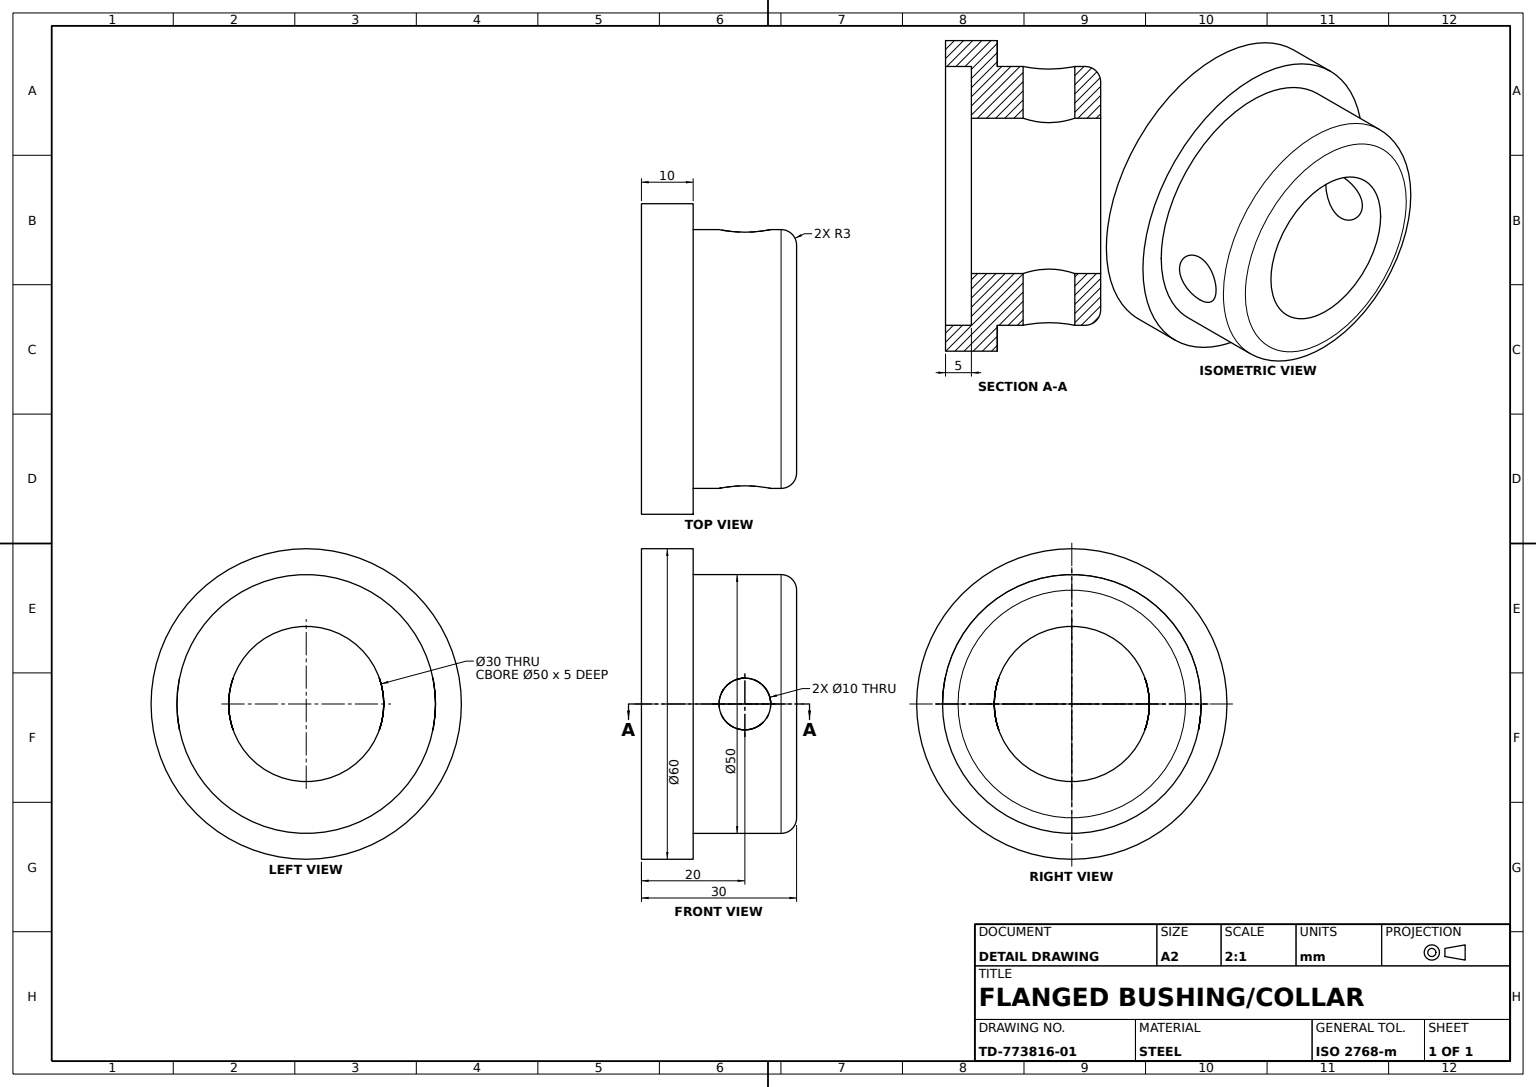
from build123d import *

# Parameters (mm, degrees)
FLANGE_PROFILE_60_R      = 30
BASE_FLANGE_60X10_DEPTH  = 10
BOSS_PROFILE_50_R        = 25
COLLAR_BOSS_50X20_DEPTH  = 20
BOSS_EDGE_FILLET_R3_R    = 3
CROSS_HOLE_PROFILE_10_R  = 5
CROSS_HOLE_10_DEPTH      = 35
COUNTERBORE_PROFILE_50_R = 25
COUNTERBORE_50X5_DEPTH   = 5
BORE_PROFILE_30_R        = 15
THROUGH_BORE_30_DEPTH    = 94


with BuildPart() as part:
    # Flange Profile Ø60 → Base Flange Ø60x10 (new body)
    with BuildSketch(Plane(origin=(0, 0, 0), x_dir=(1, 0, 0), z_dir=(0, 1, 0))):
        with Locations(Location((0, 0, 0), (0, 0, 270))):
            Circle(FLANGE_PROFILE_60_R)
    extrude(amount=BASE_FLANGE_60X10_DEPTH)

    # Boss Profile Ø50 → Collar Boss Ø50x20 (add)
    with BuildSketch(Plane(origin=(0, 10, 0), x_dir=(1, 0, 0), z_dir=(0, 1, 0))):
        with Locations(Location((0, 0, 0), (0, 0, 270))):
            Circle(BOSS_PROFILE_50_R)
    extrude(amount=COLLAR_BOSS_50X20_DEPTH)

    # Boss Edge Fillet R3
    boss_edge_fillet_r3_edges = [part.edges().sort_by_distance(p)[0] for p in [
        (0, 30, -25),
    ]]
    fillet(boss_edge_fillet_r3_edges, radius=BOSS_EDGE_FILLET_R3_R)

    # Cross Hole Profile Ø10 → Cross Hole Ø10 (cut, symmetric)
    with BuildSketch(Plane.XY):
        with Locations((0, 20)):
            Circle(CROSS_HOLE_PROFILE_10_R)
    extrude(amount=CROSS_HOLE_10_DEPTH, both=True, mode=Mode.SUBTRACT)

    # Counterbore Profile Ø50 → Counterbore Ø50x5 (cut)
    with BuildSketch(Plane.XZ):
        with Locations(Location((0, 0, 0), (0, 0, 90))):
            Circle(COUNTERBORE_PROFILE_50_R)
    extrude(amount=-COUNTERBORE_50X5_DEPTH, mode=Mode.SUBTRACT)

    # Bore Profile Ø30 → Through Bore Ø30 (cut)
    with BuildSketch(Plane.XZ.offset(-5)):
        with Locations(Location((0, 0, 0), (0, 0, 270))):
            Circle(BORE_PROFILE_30_R)
    extrude(amount=-THROUGH_BORE_30_DEPTH, mode=Mode.SUBTRACT)


solid = part.part
